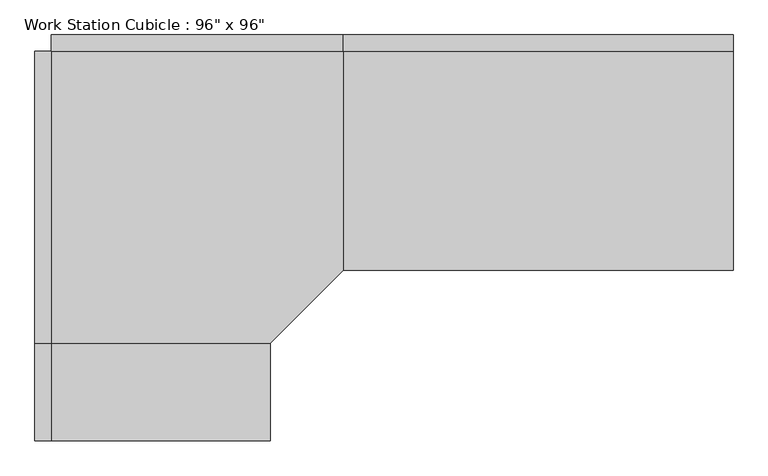
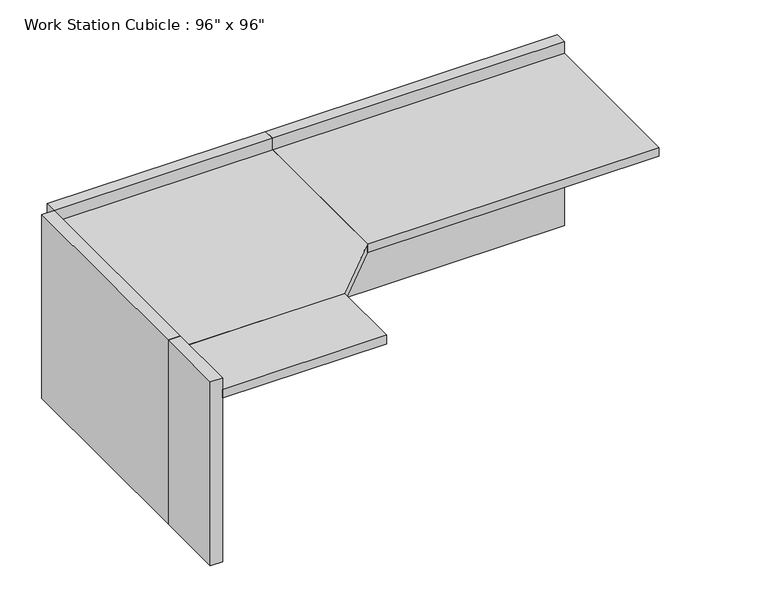
"""IFC4 building model written with IfcOpenShell, lengths in millimetres: furniture geometry."""

from ifc_helpers import new_model, si_unit, frame, origin, origin_with_axes, place, context, project, spatial, polyline, outline, extrude, source, transform, mapped, element, save


def furniture_3c9f2b99(model_context):
    return source(origin(), model_context, "Body", "SweptSolid", [
        extrude(outline(polyline([(-80.9317522, -545.8230076), (833.4682478, -545.8230076), (833.4682478, -1231.6230076), (604.8682478, -1460.2230076), (-80.9317522, -1460.2230076), (-80.9317522, -545.8230076)])), frame((0.0, 0.0, 723.9), z_axis=(0.0, 0.0, 1.0), x_axis=(1.0, 0.0, 0.0)), (0.0, 0.0, 1.0), 38.1),
        extrude(outline(polyline([(604.8682478, -1765.0230076), (-80.9317522, -1765.0230076), (-80.9317522, -1460.2230076), (604.8682478, -1460.2230076), (604.8682478, -1765.0230076)])), frame((0.0, 0.0, 723.9), z_axis=(0.0, 0.0, 1.0), x_axis=(1.0, 0.0, 0.0)), (0.0, 0.0, 1.0), 38.1),
        extrude(outline(polyline([(2052.6682478, -1231.6230076), (833.4682478, -1231.6230076), (833.4682478, -545.8230076), (2052.6682478, -545.8230076), (2052.6682478, -1231.6230076)])), frame((0.0, 0.0, 723.9), z_axis=(0.0, 0.0, 1.0), x_axis=(1.0, 0.0, 0.0)), (0.0, 0.0, 1.0), 38.1),
        extrude(outline(polyline([(2052.6682478, -545.8230076), (833.4682478, -545.8230076), (833.4682478, -495.0230076), (2052.6682478, -495.0230076), (2052.6682478, -545.8230076)])), origin_with_axes(), (0.0, 0.0, 1.0), 812.8),
        extrude(outline(polyline([(833.4682478, -545.8230076), (-80.9317522, -545.8230076), (-80.9317522, -495.0230076), (833.4682478, -495.0230076), (833.4682478, -545.8230076)])), origin_with_axes(), (0.0, 0.0, 1.0), 812.8),
        extrude(outline(polyline([(-80.9317522, -1460.2230076), (-131.7317522, -1460.2230076), (-131.7317522, -545.8230076), (-80.9317522, -545.8230076), (-80.9317522, -1460.2230076)])), origin_with_axes(), (0.0, 0.0, 1.0), 812.8),
        extrude(outline(polyline([(-80.9317522, -1765.0230076), (-131.7317522, -1765.0230076), (-131.7317522, -1460.2230076), (-80.9317522, -1460.2230076), (-80.9317522, -1765.0230076)])), origin_with_axes(), (0.0, 0.0, 1.0), 812.8),
    ])


if __name__ == "__main__":
    model = new_model("IFC4")
    model_context = context("Model", 3, world=origin())
    ifc_project = project(units=[si_unit("LENGTHUNIT", "METRE", prefix="MILLI")], contexts=[model_context])
    site = spatial("IfcSite", under=ifc_project)
    building = spatial("IfcBuilding", under=site)
    placement = place(None, origin())
    furniture_shape = furniture_3c9f2b99(model_context)
    element("IfcFurniture", 1, ObjectType="Work Station Cubicle : 96\" x 96\"", at=placement, inside=building, context=model_context, shape_type="MappedRepresentation", body=[
        mapped(furniture_shape, transform((0.0, 0.0, 0.0), x_axis=(1.0, 0.0, 0.0), y_axis=(0.0, 1.0, 0.0), z_axis=(0.0, 0.0, 1.0))),
    ])
    save(model, "model.ifc")

# Revit data of these elements
# Type "Work Station Cubicle : 96\" x 96\""
#   Assembly Code = "E2020"
#   Desktop Height = 2' - 6"
#   Desktop1 Width = 2' - 3"
#   Desktop2 Width = 2' - 3"
#   Panel Height = 2' - 8"
#   Panel1 Length = 1' - 0"
#   Panel2 Length = 4' - 0"
#   Cube Panel Material = Textile - Light Gray
#   Work Top Material = Laminate, Ivory, Matte
#   Default Elevation = 0
# Element 1 (IfcFurniture, "Work Station Cubicle : 96\" x 96\"")
#   Materials on its faces: "Textile - Light Gray", "Laminate, Ivory, Matte"
# Materials
#   "Textile - Light Gray": class "Fabric", colour RGB 204 204 204, transparency 0
#   "Laminate, Ivory, Matte": class "Plastic", colour RGB 247 247 239, transparency 0, Description = "Plastic Laminate - Ivory, Matte", Cost = 0
